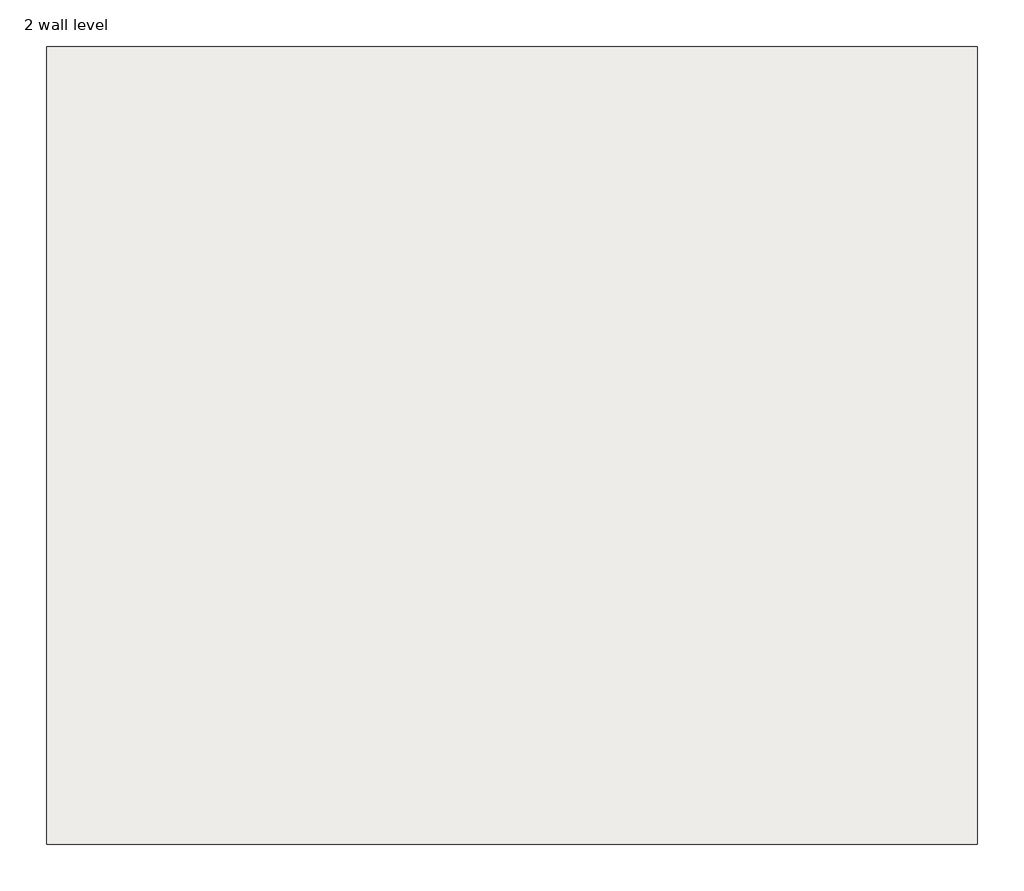
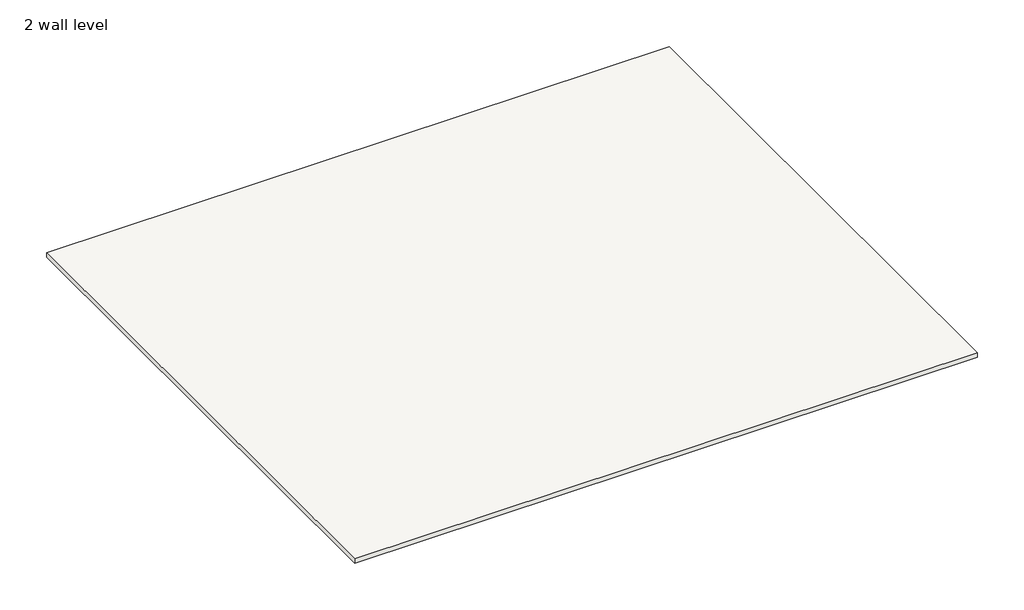
# One storey: 1 roof.
"""IFC4 building model written with IfcOpenShell, lengths in millimetres."""

from ifc_helpers import new_model, si_unit, frame, origin, place, context, project, spatial, polyline, outline, extrude, element, save

model = new_model("IFC4")

# Units and contexts
model_context = context("Model", 3, world=origin())
ifc_project = project(units=[si_unit("LENGTHUNIT", "METRE", prefix="MILLI")], contexts=[model_context])

# Site, building, storey
site = spatial("IfcSite", under=ifc_project)
building = spatial("IfcBuilding", under=site)
storey = spatial("IfcBuildingStorey", under=building, Name="2 wall level", Elevation=3505.2)

# Roof
placement = place(None, origin())
element("IfcRoof", 1, ObjectType="6\"", at=placement, inside=storey, context=model_context, shape_type="SweptSolid", body=[
    extrude(outline(polyline([(4816.0294854, -11410.7564399), (-14868.9705146, -11410.7564399), (-14868.9705146, 5454.8435601), (4816.0294854, 5454.8435601), (4816.0294854, -11410.7564399)])), frame((0.0, 0.0, 3505.2), z_axis=(0.0, 0.0, 1.0), x_axis=(1.0, 0.0, 0.0)), (0.0, 0.0, 1.0), 152.4),
])

save(model, "model.ifc")

# Revit data of these elements
# Type "6\""
#   Assembly Code = "B1020"
#   Layers, outside or top first: 0' - 6" no material (function 1)
# Element 1 (IfcRoof, "6\"")
#   built-in parameter 1001705 = 12 (stored number, unit not read)
#   built-in parameter 1001710 = 33615
#   Phase Created = New Construction
#   Materials on its faces: "Default Roof"
# Materials
#   "Default Roof": colour RGB 88 101 114, transparency 0, Cost = 0
